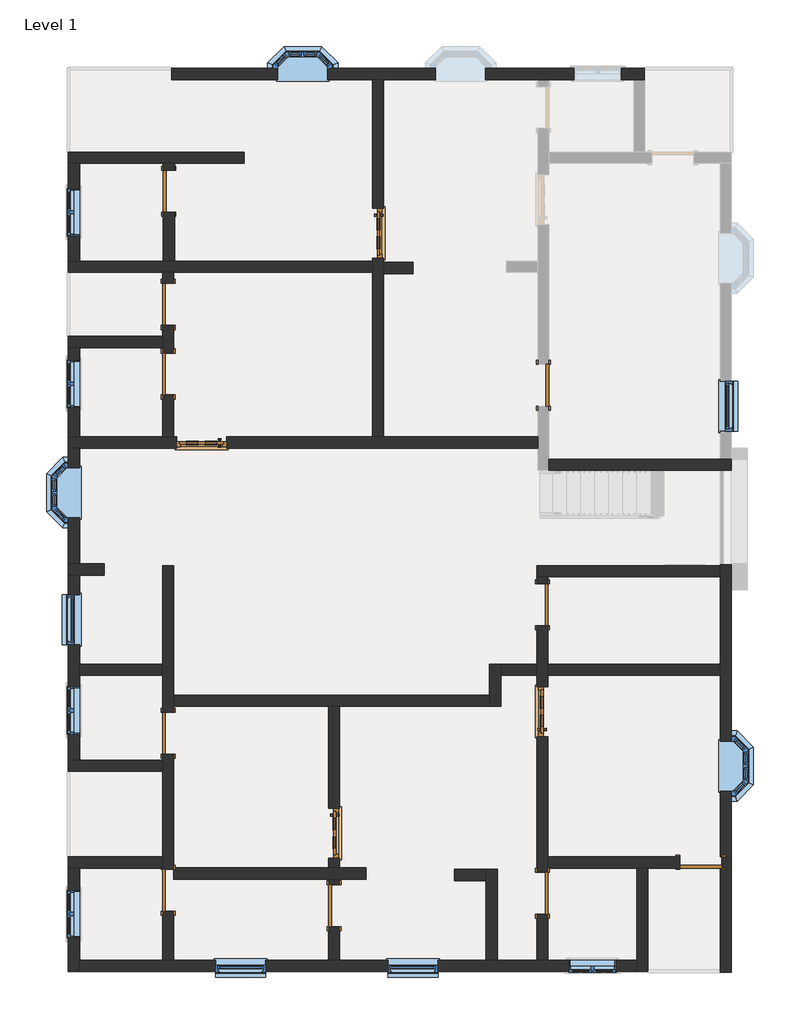
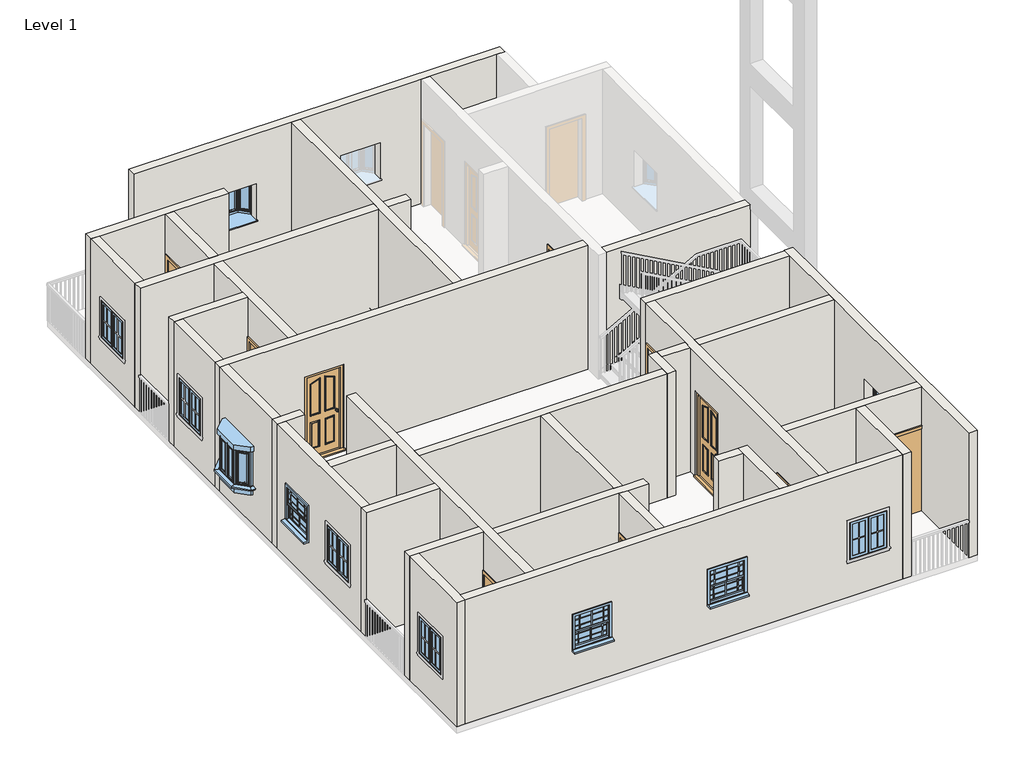
# One storey, part 1 of 4: 34 walls, 14 doors, 12 windows.
"""IFC4 building model written with IfcOpenShell, lengths in millimetres."""

from ifc_helpers import new_model, si_unit, frame, origin, origin_with_axes, place, context, project, spatial, polyline, outline, extrude, faceted_brep, transform, mapped, element, save
from components import doors_extsgl_12_910x2110mm_9a09825e, door_fadea3f2, door_53b1b562, window_910x910mm_67ef725a, window_c29befe5, windows_sash_w_bars_1_910x910mm_b688f793

model = new_model("IFC4")

# Units and contexts
model_context = context("Model", 3, world=origin())
ifc_project = project(units=[si_unit("LENGTHUNIT", "METRE", prefix="MILLI")], contexts=[model_context])

# Site, building, storey
site = spatial("IfcSite", under=ifc_project)
building = spatial("IfcBuilding", under=site)
storey = spatial("IfcBuildingStorey", under=building, Name="Level 1", Elevation=0.0)

# Doors
placement = place(None, origin())
doors_extsgl_12_910x2110mm_shape = doors_extsgl_12_910x2110mm_9a09825e(model_context)
element("IfcDoor", 1, ObjectType="Doors_ExtSgl_12 : 910x2110mm", at=placement, inside=storey, context=model_context, shape_type="MappedRepresentation", body=[
    mapped(doors_extsgl_12_910x2110mm_shape, transform((-1409.2058717, 5320.2339901, 0.0), x_axis=(0.0, -1.0, 0.0), y_axis=(1.0, 0.0, 0.0), z_axis=(0.0, 0.0, 1.0))),
])
element("IfcDoor", 2, ObjectType="Doors_ExtSgl_12 : 910x2110mm", at=placement, inside=storey, context=model_context, shape_type="MappedRepresentation", body=[
    mapped(doors_extsgl_12_910x2110mm_shape, transform((-4622.3058717, 1514.4547293, 0.0), x_axis=(-1.0, 0.0, 0.0), y_axis=(0.0, -1.0, 0.0), z_axis=(0.0, 0.0, 1.0))),
])
element("IfcDoor", 3, ObjectType="Doors_ExtSgl_12 : 910x2110mm", at=placement, inside=storey, context=model_context, shape_type="MappedRepresentation", body=[
    mapped(doors_extsgl_12_910x2110mm_shape, transform((-2209.3058717, -5597.5452707, 0.0), x_axis=(0.0, -1.0, 0.0), y_axis=(1.0, 0.0, 0.0), z_axis=(0.0, 0.0, 1.0))),
])
element("IfcDoor", 4, ObjectType="Doors_ExtSgl_12 : 910x2110mm", at=placement, inside=storey, context=model_context, shape_type="MappedRepresentation", body=[
    mapped(doors_extsgl_12_910x2110mm_shape, transform((1587.9941283, -3384.0437545, 0.0), x_axis=(0.0, 1.0, 0.0), y_axis=(-1.0, 0.0, 0.0), z_axis=(0.0, 0.0, 1.0))),
])
door_shape = door_fadea3f2(model_context)
element("IfcDoor", 5, ObjectType="Single-Flush : 30\" x 80\"", at=placement, inside=storey, context=model_context, shape_type="MappedRepresentation", body=[
    mapped(door_shape, transform((-5219.2058717, 6086.4547293, 0.0), x_axis=(0.0, 1.0, 0.0), y_axis=(-1.0, 0.0, 0.0), z_axis=(0.0, 0.0, 1.0))),
])
element("IfcDoor", 6, ObjectType="Single-Flush : 30\" x 80\"", at=placement, inside=storey, context=model_context, shape_type="MappedRepresentation", body=[
    mapped(door_shape, transform((-5231.9058717, -6637.2703483, 0.0), x_axis=(0.0, 1.0, 0.0), y_axis=(-1.0, 0.0, 0.0), z_axis=(0.0, 0.0, 1.0))),
])
element("IfcDoor", 7, ObjectType="Single-Flush : 30\" x 80\"", at=placement, inside=storey, context=model_context, shape_type="MappedRepresentation", body=[
    mapped(door_shape, transform((-2209.3058717, -6918.3452707, 0.0), x_axis=(0.0, 1.0, 0.0), y_axis=(-1.0, 0.0, 0.0), z_axis=(0.0, 0.0, 1.0))),
])
door_2_shape = door_53b1b562(model_context)
element("IfcDoor", 8, ObjectType="Single-Flush : 30\" x 80\"", at=placement, inside=storey, context=model_context, shape_type="MappedRepresentation", body=[
    mapped(door_2_shape, transform((-5231.9058717, 2759.0547293, 0.0), x_axis=(0.0, -1.0, 0.0), y_axis=(1.0, 0.0, 0.0), z_axis=(0.0, 0.0, 1.0))),
])
element("IfcDoor", 9, ObjectType="Single-Flush : 30\" x 80\"", at=placement, inside=storey, context=model_context, shape_type="MappedRepresentation", body=[
    mapped(door_2_shape, transform((-5231.9058717, -3778.816952, 0.0), x_axis=(0.0, -1.0, 0.0), y_axis=(1.0, 0.0, 0.0), z_axis=(0.0, 0.0, 1.0))),
])
element("IfcDoor", 10, ObjectType="Single-Flush : 30\" x 80\"", at=placement, inside=storey, context=model_context, shape_type="MappedRepresentation", body=[
    mapped(door_2_shape, transform((1587.9941283, -6689.7452707, 0.0), x_axis=(0.0, 1.0, 0.0), y_axis=(-1.0, 0.0, 0.0), z_axis=(0.0, 0.0, 1.0))),
])
element("IfcDoor", 11, ObjectType="Single-Flush : 30\" x 80\"", at=placement, inside=storey, context=model_context, shape_type="MappedRepresentation", body=[
    mapped(door_2_shape, transform((4470.8941283, -6130.9452707, 0.0), x_axis=(1.0, 0.0, 0.0), y_axis=(0.0, 1.0, 0.0), z_axis=(0.0, 0.0, 1.0))),
])
element("IfcDoor", 12, ObjectType="Single-Flush : 30\" x 80\"", at=placement, inside=storey, context=model_context, shape_type="MappedRepresentation", body=[
    mapped(door_2_shape, transform((1587.9941283, -1440.3867138, 0.0), x_axis=(0.0, 1.0, 0.0), y_axis=(-1.0, 0.0, 0.0), z_axis=(0.0, 0.0, 1.0))),
])
element("IfcDoor", 13, ObjectType="Single-Flush : 30\" x 80\"", at=placement, inside=storey, context=model_context, shape_type="MappedRepresentation", body=[
    mapped(door_2_shape, transform((1600.6941283, 2555.8547293, 0.0), x_axis=(0.0, 1.0, 0.0), y_axis=(-1.0, 0.0, 0.0), z_axis=(0.0, 0.0, 1.0))),
])
element("IfcDoor", 14, ObjectType="Single-Flush : 30\" x 80\"", at=placement, inside=storey, context=model_context, shape_type="MappedRepresentation", body=[
    mapped(door_2_shape, transform((-5231.9058717, 4026.9443597, 0.0), x_axis=(0.0, -1.0, 0.0), y_axis=(1.0, 0.0, 0.0), z_axis=(0.0, 0.0, 1.0))),
])

# Walls
element("IfcWall", 15, ObjectType="Generic - 4.5\"", at=placement, inside=storey, context=model_context, shape_type="Brep", body=[
    faceted_brep([(-1510.8058717, 4865.2339901, 2110.0), (-1510.8058717, 4865.2339901, 0.0), (-1510.8058717, 4812.2339901, 0.0), (-1510.8058717, 4609.0339901, 0.0), (-1510.8058717, 1616.0547293, 0.0), (-1510.8058717, 1616.0547293, 3048.0), (-1510.8058717, 4609.0339901, 3048.0), (-1510.8058717, 4812.2339901, 3048.0), (-1510.8058717, 8118.4547293, 3048.0), (-1510.8058717, 8118.4547293, 0.0), (-1510.8058717, 5775.2339901, 0.0), (-1510.8058717, 5775.2339901, 2110.0), (-1307.6058717, 1616.0547293, 0.0), (-1307.6058717, 4587.8547293, 0.0), (-1307.6058717, 4791.0547293, 0.0), (-1307.6058717, 4865.2339901, 0.0), (-1307.6058717, 4865.2339901, 2110.0), (-1307.6058717, 5775.2339901, 2110.0), (-1307.6058717, 5775.2339901, 0.0), (-1307.6058717, 8118.4547293, 0.0), (-1307.6058717, 8118.4547293, 3048.0), (-1307.6058717, 4791.0547293, 3048.0), (-1307.6058717, 4587.8547293, 3048.0), (-1307.6058717, 1616.0547293, 3048.0)], [[[0, 1, 2, 3, 4, 5, 6, 7, 8, 9, 10, 11]], [[12, 13, 14, 15, 16, 17, 18, 19, 20, 21, 22, 23]], [[10, 9, 19, 18]], [[4, 3, 2, 1, 15, 14, 13, 12]], [[8, 7, 6, 5, 23, 22, 21, 20]], [[9, 8, 20, 19]], [[5, 4, 12, 23]], [[18, 17, 11, 10]], [[16, 15, 1, 0]], [[17, 16, 0, 11]]]),
])
element("IfcWall", 16, ObjectType="Generic - 4.5\"", at=placement, inside=storey, context=model_context, shape_type="Brep", body=[
    faceted_brep([(-7048.0058717, 4609.0339901, 0.0), (-5333.5058717, 4609.0339901, 0.0), (-5130.3058717, 4609.0339901, 0.0), (-1510.8058717, 4609.0339901, 0.0), (-1510.8058717, 4609.0339901, 3048.0), (-5130.3058717, 4609.0339901, 3048.0), (-5333.5058717, 4609.0339901, 3048.0), (-7048.0058717, 4609.0339901, 3048.0), (-7048.0058717, 4812.2339901, 0.0), (-7048.0058717, 4812.2339901, 3048.0), (-6844.8058717, 4812.2339901, 3048.0), (-5320.8058717, 4812.2339901, 3048.0), (-5117.6058717, 4812.2339901, 3048.0), (-1510.8058717, 4812.2339901, 3048.0), (-1510.8058717, 4812.2339901, 0.0), (-5117.6058717, 4812.2339901, 0.0), (-5320.8058717, 4812.2339901, 0.0), (-6844.8058717, 4812.2339901, 0.0)], [[[0, 1, 2, 3, 4, 5, 6, 7]], [[8, 9, 10, 11, 12, 13, 14, 15, 16, 17]], [[3, 2, 1, 0, 8, 17, 16, 15, 14]], [[7, 6, 5, 4, 13, 12, 11, 10, 9]], [[4, 3, 14, 13]], [[0, 7, 9, 8]]]),
])
element("IfcWall", 17, ObjectType="Generic - 4.5\"", at=placement, inside=storey, context=model_context, shape_type="Brep", body=[
    faceted_brep([(-5333.5058717, 3645.9443597, 2032.0), (-5333.5058717, 3645.9443597, 0.0), (-5333.5058717, 3444.8547293, 0.0), (-5333.5058717, 3241.6547293, 0.0), (-5333.5058717, 3140.0547293, 0.0), (-5333.5058717, 3140.0547293, 2032.0), (-5333.5058717, 2378.0547293, 2032.0), (-5333.5058717, 2378.0547293, 0.0), (-5333.5058717, 1616.0547293, 0.0), (-5333.5058717, 1616.0547293, 3048.0), (-5333.5058717, 3241.6547293, 3048.0), (-5333.5058717, 3444.8547293, 3048.0), (-5333.5058717, 4609.0339901, 3048.0), (-5333.5058717, 4609.0339901, 0.0), (-5333.5058717, 4407.9443597, 0.0), (-5333.5058717, 4407.9443597, 2032.0), (-5130.3058717, 3140.0547293, 0.0), (-5130.3058717, 3645.9443597, 0.0), (-5130.3058717, 3645.9443597, 2032.0), (-5130.3058717, 4407.9443597, 2032.0), (-5130.3058717, 4407.9443597, 0.0), (-5130.3058717, 4609.0339901, 0.0), (-5130.3058717, 4609.0339901, 3048.0), (-5130.3058717, 1616.0547293, 3048.0), (-5130.3058717, 1616.0547293, 0.0), (-5130.3058717, 2378.0547293, 0.0), (-5130.3058717, 2378.0547293, 2032.0), (-5130.3058717, 3140.0547293, 2032.0)], [[[0, 1, 2, 3, 4, 5, 6, 7, 8, 9, 10, 11, 12, 13, 14, 15]], [[16, 17, 18, 19, 20, 21, 22, 23, 24, 25, 26, 27]], [[8, 7, 25, 24]], [[14, 13, 21, 20]], [[4, 3, 2, 1, 17, 16]], [[12, 11, 10, 9, 23, 22]], [[13, 12, 22, 21]], [[9, 8, 24, 23]], [[26, 25, 7, 6]], [[27, 26, 6, 5]], [[16, 27, 5, 4]], [[18, 17, 1, 0]], [[19, 18, 0, 15]], [[20, 19, 15, 14]]]),
])
element("IfcWall", 18, ObjectType="Generic - 4.5\"", at=placement, inside=storey, context=model_context, shape_type="Brep", body=[
    faceted_brep([(-5130.3058717, -6256.2703483, 2032.0), (-5130.3058717, -6256.2703483, 0.0), (-5130.3058717, -6230.8703483, 0.0), (-5130.3058717, -4159.816952, 0.0), (-5130.3058717, -4159.816952, 2032.0), (-5130.3058717, -3397.816952, 2032.0), (-5130.3058717, -3397.816952, 0.0), (-5130.3058717, -3286.1452707, 0.0), (-5130.3058717, -3082.9452707, 0.0), (-5130.3058717, -733.4452707, 0.0), (-5130.3058717, -733.4452707, 3048.0), (-5130.3058717, -3082.9452707, 3048.0), (-5130.3058717, -3286.1452707, 3048.0), (-5130.3058717, -6230.8703483, 3048.0), (-5130.3058717, -6434.0703483, 3048.0), (-5130.3058717, -7908.9452707, 3048.0), (-5130.3058717, -7908.9452707, 0.0), (-5130.3058717, -7018.2703483, 0.0), (-5130.3058717, -7018.2703483, 2032.0), (-5333.5058717, -4159.816952, 0.0), (-5333.5058717, -4271.4886333, 0.0), (-5333.5058717, -4474.6886333, 0.0), (-5333.5058717, -6029.3452707, 0.0), (-5333.5058717, -6232.5452707, 0.0), (-5333.5058717, -6256.2703483, 0.0), (-5333.5058717, -6256.2703483, 2032.0), (-5333.5058717, -7018.2703483, 2032.0), (-5333.5058717, -7018.2703483, 0.0), (-5333.5058717, -7908.9452707, 0.0), (-5333.5058717, -7908.9452707, 3048.0), (-5333.5058717, -6232.5452707, 3048.0), (-5333.5058717, -6029.3452707, 3048.0), (-5333.5058717, -4474.6886333, 3048.0), (-5333.5058717, -4271.4886333, 3048.0), (-5333.5058717, -2727.3452707, 3048.0), (-5333.5058717, -2524.1452707, 3048.0), (-5333.5058717, -733.4452707, 3048.0), (-5333.5058717, -733.4452707, 0.0), (-5333.5058717, -2524.1452707, 0.0), (-5333.5058717, -2727.3452707, 0.0), (-5333.5058717, -3397.816952, 0.0), (-5333.5058717, -3397.816952, 2032.0), (-5333.5058717, -4159.816952, 2032.0)], [[[0, 1, 2, 3, 4, 5, 6, 7, 8, 9, 10, 11, 12, 13, 14, 15, 16, 17, 18]], [[19, 20, 21, 22, 23, 24, 25, 26, 27, 28, 29, 30, 31, 32, 33, 34, 35, 36, 37, 38, 39, 40, 41, 42]], [[40, 39, 38, 37, 9, 8, 7, 6]], [[17, 16, 28, 27]], [[3, 2, 1, 24, 23, 22, 21, 20, 19]], [[10, 9, 37, 36]], [[15, 14, 13, 12, 11, 10, 36, 35, 34, 33, 32, 31, 30, 29]], [[4, 3, 19, 42]], [[5, 4, 42, 41]], [[6, 5, 41, 40]], [[25, 24, 1, 0]], [[26, 25, 0, 18]], [[27, 26, 18, 17]], [[16, 15, 29, 28]]]),
])
element("IfcWall", 19, ObjectType="Generic - 4.5\"", at=placement, inside=storey, context=model_context, shape_type="Brep", body=[
    faceted_brep([(-7048.0058717, -898.5452707, 0.0), (-6844.8058717, -898.5452707, 0.0), (-6400.7404065, -898.5452707, 0.0), (-6400.7404065, -898.5452707, 3048.0), (-6844.8058717, -898.5452707, 3048.0), (-7048.0058717, -898.5452707, 3048.0), (-7048.0058717, -695.3452707, 0.0), (-7048.0058717, -695.3452707, 3048.0), (-6844.8058717, -695.3452707, 3048.0), (-6400.7404065, -695.3452707, 3048.0), (-6400.7404065, -695.3452707, 0.0), (-6844.8058717, -695.3452707, 0.0)], [[[0, 1, 2, 3, 4, 5]], [[6, 7, 8, 9, 10, 11]], [[2, 1, 0, 6, 11, 10]], [[3, 2, 10, 9]], [[5, 4, 3, 9, 8, 7]], [[0, 5, 7, 6]]]),
])
element("IfcWall", 20, ObjectType="Generic - 4.5\"", at=placement, inside=storey, context=model_context, shape_type="Brep", body=[
    faceted_brep([(-7048.0058717, 6594.4547293, 0.0), (-6844.8058717, 6594.4547293, 0.0), (-5320.8058717, 6594.4547293, 0.0), (-5117.6058717, 6594.4547293, 0.0), (-3847.6058717, 6594.4547293, 0.0), (-3847.6058717, 6594.4547293, 3048.0), (-5117.6058717, 6594.4547293, 3048.0), (-5320.8058717, 6594.4547293, 3048.0), (-6844.8058717, 6594.4547293, 3048.0), (-7048.0058717, 6594.4547293, 3048.0), (-7048.0058717, 6797.6547293, 0.0), (-7048.0058717, 6797.6547293, 3048.0), (-3847.6058717, 6797.6547293, 3048.0), (-3847.6058717, 6797.6547293, 0.0)], [[[0, 1, 2, 3, 4, 5, 6, 7, 8, 9]], [[10, 11, 12, 13]], [[4, 3, 2, 1, 0, 10, 13]], [[5, 4, 13, 12]], [[9, 8, 7, 6, 5, 12, 11]], [[0, 9, 11, 10]]]),
])
element("IfcWall", 21, ObjectType="Generic - 4.5\"", at=placement, inside=storey, context=model_context, shape_type="Brep", body=[
    faceted_brep([(-7048.0058717, 3241.6547293, 0.0), (-6844.8058717, 3241.6547293, 0.0), (-5333.5058717, 3241.6547293, 0.0), (-5333.5058717, 3241.6547293, 3048.0), (-6844.8058717, 3241.6547293, 3048.0), (-7048.0058717, 3241.6547293, 3048.0), (-7048.0058717, 3444.8547293, 0.0), (-7048.0058717, 3444.8547293, 3048.0), (-5333.5058717, 3444.8547293, 3048.0), (-5333.5058717, 3444.8547293, 0.0)], [[[0, 1, 2, 3, 4, 5]], [[6, 7, 8, 9]], [[2, 1, 0, 6, 9]], [[5, 4, 3, 8, 7]], [[3, 2, 9, 8]], [[0, 5, 7, 6]]]),
])
element("IfcWall", 22, ObjectType="Generic - 4.5\"", at=placement, inside=storey, context=model_context, shape_type="Brep", body=[
    faceted_brep([(-7048.0058717, 1412.8547293, 0.0), (-6844.8058717, 1412.8547293, 0.0), (-5077.3058717, 1412.8547293, 0.0), (-5077.3058717, 1412.8547293, 2110.0), (-4167.3058717, 1412.8547293, 2110.0), (-4167.3058717, 1412.8547293, 0.0), (1499.0941283, 1412.8547293, 0.0), (1499.0941283, 1412.8547293, 3048.0), (-6844.8058717, 1412.8547293, 3048.0), (-7048.0058717, 1412.8547293, 3048.0), (-5077.3058717, 1616.0547293, 2110.0), (-5077.3058717, 1616.0547293, 0.0), (-5130.3058717, 1616.0547293, 0.0), (-5333.5058717, 1616.0547293, 0.0), (-6844.8058717, 1616.0547293, 0.0), (-7048.0058717, 1616.0547293, 0.0), (-7048.0058717, 1616.0547293, 3048.0), (-6844.8058717, 1616.0547293, 3048.0), (-5333.5058717, 1616.0547293, 3048.0), (-5130.3058717, 1616.0547293, 3048.0), (-1510.8058717, 1616.0547293, 3048.0), (-1307.6058717, 1616.0547293, 3048.0), (1499.0941283, 1616.0547293, 3048.0), (1499.0941283, 1616.0547293, 0.0), (-1307.6058717, 1616.0547293, 0.0), (-1510.8058717, 1616.0547293, 0.0), (-4167.3058717, 1616.0547293, 0.0), (-4167.3058717, 1616.0547293, 2110.0)], [[[0, 1, 2, 3, 4, 5, 6, 7, 8, 9]], [[10, 11, 12, 13, 14, 15, 16, 17, 18, 19, 20, 21, 22, 23, 24, 25, 26, 27]], [[26, 25, 24, 23, 6, 5]], [[15, 14, 13, 12, 11, 2, 1, 0]], [[9, 8, 7, 22, 21, 20, 19, 18, 17, 16]], [[7, 6, 23, 22]], [[5, 4, 27, 26]], [[3, 2, 11, 10]], [[4, 3, 10, 27]], [[0, 9, 16, 15]]]),
])
element("IfcWall", 23, ObjectType="Generic - 4.5\"", at=placement, inside=storey, context=model_context, shape_type="Brep", body=[
    faceted_brep([(1702.2941283, 1006.4547293, 0.0), (5029.6941283, 1006.4547293, 0.0), (5029.6941283, 1006.4547293, 3048.0), (1702.2941283, 1006.4547293, 3048.0), (1702.2941283, 1209.6547293, 0.0), (1702.2941283, 1209.6547293, 3048.0), (4826.4941283, 1209.6547293, 3048.0), (5029.6941283, 1209.6547293, 3048.0), (5029.6941283, 1209.6547293, 0.0), (4826.4941283, 1209.6547293, 0.0)], [[[0, 1, 2, 3]], [[4, 5, 6, 7, 8, 9]], [[1, 0, 4, 9, 8]], [[3, 2, 7, 6, 5]], [[0, 3, 5, 4]], [[2, 1, 8, 7]]]),
])
element("IfcWall", 24, ObjectType="Generic - 4.5\"", at=placement, inside=storey, context=model_context, shape_type="Brep", body=[
    faceted_brep([(1486.3941283, -932.3867138, 0.0), (1689.5941283, -932.3867138, 0.0), (4826.4941283, -932.3867138, 0.0), (4826.4941283, -932.3867138, 3048.0), (1689.5941283, -932.3867138, 3048.0), (1486.3941283, -932.3867138, 3048.0), (1486.3941283, -729.1867138, 0.0), (1486.3941283, -729.1867138, 3048.0), (4826.4941283, -729.1867138, 3048.0), (4826.4941283, -729.1867138, 0.0)], [[[0, 1, 2, 3, 4, 5]], [[6, 7, 8, 9]], [[2, 1, 0, 6, 9]], [[5, 4, 3, 8, 7]], [[3, 2, 9, 8]], [[0, 5, 7, 6]]]),
])
element("IfcWall", 25, ObjectType="Generic - 4.5\"", at=placement, inside=storey, context=model_context, shape_type="Brep", body=[
    faceted_brep([(1486.3941283, -932.3867138, 0.0), (1486.3941283, -1059.3867138, 0.0), (1486.3941283, -1059.3867138, 2032.0), (1486.3941283, -1821.3867138, 2032.0), (1486.3941283, -1821.3867138, 0.0), (1486.3941283, -2520.4437545, 0.0), (1486.3941283, -2723.6437545, 0.0), (1486.3941283, -2929.0437545, 0.0), (1486.3941283, -2929.0437545, 2110.0), (1486.3941283, -3839.0437545, 2110.0), (1486.3941283, -3839.0437545, 0.0), (1486.3941283, -6308.7452707, 0.0), (1486.3941283, -6308.7452707, 2032.0), (1486.3941283, -7070.7452707, 2032.0), (1486.3941283, -7070.7452707, 0.0), (1486.3941283, -7908.9452707, 0.0), (1486.3941283, -7908.9452707, 3048.0), (1486.3941283, -2723.6437545, 3048.0), (1486.3941283, -2520.4437545, 3048.0), (1486.3941283, -932.3867138, 3048.0), (1689.5941283, -1059.3867138, 2032.0), (1689.5941283, -1059.3867138, 0.0), (1689.5941283, -932.3867138, 0.0), (1689.5941283, -932.3867138, 3048.0), (1689.5941283, -2520.4437545, 3048.0), (1689.5941283, -2723.6437545, 3048.0), (1689.5941283, -6029.3452707, 3048.0), (1689.5941283, -6232.5452707, 3048.0), (1689.5941283, -7908.9452707, 3048.0), (1689.5941283, -7908.9452707, 0.0), (1689.5941283, -7070.7452707, 0.0), (1689.5941283, -7070.7452707, 2032.0), (1689.5941283, -6308.7452707, 2032.0), (1689.5941283, -6308.7452707, 0.0), (1689.5941283, -6232.5452707, 0.0), (1689.5941283, -6029.3452707, 0.0), (1689.5941283, -3839.0437545, 0.0), (1689.5941283, -3839.0437545, 2110.0), (1689.5941283, -2929.0437545, 2110.0), (1689.5941283, -2929.0437545, 0.0), (1689.5941283, -2723.6437545, 0.0), (1689.5941283, -2520.4437545, 0.0), (1689.5941283, -1821.3867138, 0.0), (1689.5941283, -1821.3867138, 2032.0)], [[[0, 1, 2, 3, 4, 5, 6, 7, 8, 9, 10, 11, 12, 13, 14, 15, 16, 17, 18, 19]], [[20, 21, 22, 23, 24, 25, 26, 27, 28, 29, 30, 31, 32, 33, 34, 35, 36, 37, 38, 39, 40, 41, 42, 43]], [[30, 29, 15, 14]], [[36, 35, 34, 33, 11, 10]], [[22, 21, 1, 0]], [[42, 41, 40, 39, 7, 6, 5, 4]], [[19, 18, 17, 16, 28, 27, 26, 25, 24, 23]], [[0, 19, 23, 22]], [[10, 9, 37, 36]], [[8, 7, 39, 38]], [[9, 8, 38, 37]], [[12, 11, 33, 32]], [[13, 12, 32, 31]], [[14, 13, 31, 30]], [[2, 1, 21, 20]], [[3, 2, 20, 43]], [[4, 3, 43, 42]], [[16, 15, 29, 28]]]),
])
element("IfcWall", 26, ObjectType="Generic - 4.5\"", at=placement, inside=storey, context=model_context, shape_type="SweptSolid", body=[
    extrude(outline(polyline([(4826.4941283, -2723.6437545), (1689.5941283, -2723.6437545), (1689.5941283, -2520.4437545), (4826.4941283, -2520.4437545), (4826.4941283, -2723.6437545)])), origin_with_axes(), (0.0, 0.0, 1.0), 3048.0),
])
element("IfcWall", 27, ObjectType="Generic - 4.5\"", at=placement, inside=storey, context=model_context, shape_type="Brep", body=[
    faceted_brep([(4826.4941283, -6232.5452707, 3048.0), (3505.6941283, -6232.5452707, 3048.0), (3302.4941283, -6232.5452707, 3048.0), (1689.5941283, -6232.5452707, 3048.0), (1689.5941283, -6232.5452707, 0.0), (3302.4941283, -6232.5452707, 0.0), (3505.6941283, -6232.5452707, 0.0), (4089.8941283, -6232.5452707, 0.0), (4089.8941283, -6232.5452707, 2032.0), (4826.4941283, -6232.5452707, 2032.0), (1689.5941283, -6029.3452707, 3048.0), (4826.4941283, -6029.3452707, 3048.0), (4826.4941283, -6029.3452707, 2032.0), (4089.8941283, -6029.3452707, 2032.0), (4089.8941283, -6029.3452707, 0.0), (1689.5941283, -6029.3452707, 0.0)], [[[0, 1, 2, 3, 4, 5, 6, 7, 8, 9]], [[10, 11, 12, 13, 14, 15]], [[4, 15, 14, 7, 6, 5]], [[3, 2, 1, 0, 11, 10]], [[11, 0, 9, 12]], [[4, 3, 10, 15]], [[8, 13, 12, 9]], [[13, 8, 7, 14]]]),
])
element("IfcWall", 28, ObjectType="Generic - 4.5\"", at=placement, inside=storey, context=model_context, shape_type="Brep", body=[
    faceted_brep([(3302.4941283, -6232.5452707, 0.0), (3302.4941283, -7908.9452707, 0.0), (3302.4941283, -8112.1452707, 0.0), (3302.4941283, -8112.1452707, 3048.0), (3302.4941283, -7908.9452707, 3048.0), (3302.4941283, -6232.5452707, 3048.0), (3505.6941283, -6232.5452707, 0.0), (3505.6941283, -6232.5452707, 3048.0), (3505.6941283, -8112.1452707, 3048.0), (3505.6941283, -8112.1452707, 0.0)], [[[0, 1, 2, 3, 4, 5]], [[6, 7, 8, 9]], [[2, 1, 0, 6, 9]], [[5, 4, 3, 8, 7]], [[0, 5, 7, 6]], [[3, 2, 9, 8]]]),
])
element("IfcWall", 29, ObjectType="Generic - 4.5\"", at=placement, inside=storey, context=model_context, shape_type="SweptSolid", body=[
    extrude(outline(polyline([(-5333.5058717, -2727.3452707), (-6844.8058717, -2727.3452707), (-6844.8058717, -2524.1452707), (-5333.5058717, -2524.1452707), (-5333.5058717, -2727.3452707)])), origin_with_axes(), (0.0, 0.0, 1.0), 3048.0),
])
element("IfcWall", 30, ObjectType="Generic - 4.5\"", at=placement, inside=storey, context=model_context, shape_type="Brep", body=[
    faceted_brep([(-7048.0058717, -4474.6886333, 0.0), (-5333.5058717, -4474.6886333, 0.0), (-5333.5058717, -4474.6886333, 3048.0), (-7048.0058717, -4474.6886333, 3048.0), (-7048.0058717, -4271.4886333, 0.0), (-7048.0058717, -4271.4886333, 3048.0), (-6844.8058717, -4271.4886333, 3048.0), (-5333.5058717, -4271.4886333, 3048.0), (-5333.5058717, -4271.4886333, 0.0), (-6844.8058717, -4271.4886333, 0.0)], [[[0, 1, 2, 3]], [[4, 5, 6, 7, 8, 9]], [[1, 0, 4, 9, 8]], [[3, 2, 7, 6, 5]], [[2, 1, 8, 7]], [[0, 3, 5, 4]]]),
])
element("IfcWall", 31, ObjectType="Generic - 4.5\"", at=placement, inside=storey, context=model_context, shape_type="Brep", body=[
    faceted_brep([(-7048.0058717, -6232.5452707, 0.0), (-6844.8058717, -6232.5452707, 0.0), (-5333.5058717, -6232.5452707, 0.0), (-5333.5058717, -6232.5452707, 3048.0), (-6844.8058717, -6232.5452707, 3048.0), (-7048.0058717, -6232.5452707, 3048.0), (-7048.0058717, -6029.3452707, 0.0), (-7048.0058717, -6029.3452707, 3048.0), (-5333.5058717, -6029.3452707, 3048.0), (-5333.5058717, -6029.3452707, 0.0)], [[[0, 1, 2, 3, 4, 5]], [[6, 7, 8, 9]], [[2, 1, 0, 6, 9]], [[5, 4, 3, 8, 7]], [[3, 2, 9, 8]], [[0, 5, 7, 6]]]),
])
element("IfcWall", 32, ObjectType="Generic - 4.5\"", at=placement, inside=storey, context=model_context, shape_type="Brep", body=[
    faceted_brep([(-5130.3058717, -6434.0703483, 0.0), (-2310.9058717, -6434.0703483, 0.0), (-2107.7058717, -6434.0703483, 0.0), (-1625.1058717, -6434.0703483, 0.0), (-1625.1058717, -6434.0703483, 3048.0), (-2107.7058717, -6434.0703483, 3048.0), (-2310.9058717, -6434.0703483, 3048.0), (-5130.3058717, -6434.0703483, 3048.0), (-5130.3058717, -6230.8703483, 0.0), (-5130.3058717, -6230.8703483, 3048.0), (-2310.9058717, -6230.8703483, 3048.0), (-2107.7058717, -6230.8703483, 3048.0), (-1625.1058717, -6230.8703483, 3048.0), (-1625.1058717, -6230.8703483, 0.0), (-2107.7058717, -6230.8703483, 0.0), (-2310.9058717, -6230.8703483, 0.0), (-5130.3058717, -6256.2703483, 0.0)], [[[0, 1, 2, 3, 4, 5, 6, 7]], [[8, 9, 10, 11, 12, 13, 14, 15]], [[3, 2, 1, 0, 16, 8, 15, 14, 13]], [[4, 3, 13, 12]], [[7, 6, 5, 4, 12, 11, 10, 9]], [[0, 7, 9, 8, 16]]]),
])
element("IfcWall", 33, ObjectType="Generic - 4.5\"", at=placement, inside=storey, context=model_context, shape_type="Brep", body=[
    faceted_brep([(762.4941283, -7908.9452707, 0.0), (762.4941283, -6257.9452707, 0.0), (762.4941283, -6257.9452707, 3048.0), (762.4941283, -7908.9452707, 3048.0), (559.2941283, -7908.9452707, 0.0), (559.2941283, -7908.9452707, 3048.0), (559.2941283, -6461.1452707, 3048.0), (559.2941283, -6257.9452707, 3048.0), (559.2941283, -6257.9452707, 0.0), (559.2941283, -6461.1452707, 0.0)], [[[0, 1, 2, 3]], [[4, 5, 6, 7, 8, 9]], [[1, 0, 4, 9, 8]], [[3, 2, 7, 6, 5]], [[2, 1, 8, 7]], [[0, 3, 5, 4]]]),
])
element("IfcWall", 34, ObjectType="Generic - 4.5\"", at=placement, inside=storey, context=model_context, shape_type="SweptSolid", body=[
    extrude(outline(polyline([(-12.2058717, -6257.9452707), (559.2941283, -6257.9452707), (559.2941283, -6461.1452707), (-12.2058717, -6461.1452707), (-12.2058717, -6257.9452707)])), origin_with_axes(), (0.0, 0.0, 1.0), 3048.0),
])
element("IfcWall", 35, ObjectType="Generic - 4.5\"", at=placement, inside=storey, context=model_context, shape_type="SweptSolid", body=[
    extrude(outline(polyline([(-3286.1452707, 3048.0), (-3286.1452707, 0.0), (-5142.5452707, 0.0), (-5142.5452707, 2110.0), (-6052.5452707, 2110.0), (-6052.5452707, 0.0), (-6230.8703483, 0.0), (-6230.8703483, 3048.0), (-3286.1452707, 3048.0)])), frame((-2310.9058717, 0.0, 0.0), z_axis=(1.0, 0.0, 0.0), x_axis=(0.0, 1.0, 0.0)), (0.0, 0.0, 1.0), 203.2),
    extrude(outline(polyline([(-6537.3452707, 0.0), (-6537.3452707, 2032.0), (-7299.3452707, 2032.0), (-7299.3452707, 0.0), (-7908.9452707, 0.0), (-7908.9452707, 3048.0), (-6434.0703483, 3048.0), (-6434.0703483, 0.0), (-6537.3452707, 0.0)])), frame((-2310.9058717, 0.0, 0.0), z_axis=(1.0, 0.0, 0.0), x_axis=(0.0, 1.0, 0.0)), (0.0, 0.0, 1.0), 203.2),
])
element("IfcWall", 36, ObjectType="Generic - 4.5\"", at=placement, inside=storey, context=model_context, shape_type="Brep", body=[
    faceted_brep([(-5130.3058717, -3286.1452707, 0.0), (-2310.9058717, -3286.1452707, 0.0), (-2107.7058717, -3286.1452707, 0.0), (622.0199378, -3286.1452707, 0.0), (622.0199378, -3286.1452707, 3048.0), (-2107.7058717, -3286.1452707, 3048.0), (-2310.9058717, -3286.1452707, 3048.0), (-5130.3058717, -3286.1452707, 3048.0), (-5130.3058717, -3082.9452707, 0.0), (-5130.3058717, -3082.9452707, 3048.0), (622.0199378, -3082.9452707, 3048.0), (622.0199378, -3082.9452707, 0.0)], [[[0, 1, 2, 3, 4, 5, 6, 7]], [[8, 9, 10, 11]], [[3, 2, 1, 0, 8, 11]], [[7, 6, 5, 4, 10, 9]], [[0, 7, 9, 8]], [[4, 3, 11, 10]]]),
])
element("IfcWall", 37, ObjectType="Generic - 4.5\"", at=placement, inside=storey, context=model_context, shape_type="Brep", body=[
    faceted_brep([(825.2199378, -3286.1452707, 0.0), (825.2199378, -2723.6437545, 0.0), (825.2199378, -2520.4437545, 0.0), (825.2199378, -2520.4437545, 3048.0), (825.2199378, -2723.6437545, 3048.0), (825.2199378, -3286.1452707, 3048.0), (622.0199378, -3286.1452707, 0.0), (622.0199378, -3286.1452707, 3048.0), (622.0199378, -3082.9452707, 3048.0), (622.0199378, -2520.4437545, 3048.0), (622.0199378, -2520.4437545, 0.0), (622.0199378, -3082.9452707, 0.0)], [[[0, 1, 2, 3, 4, 5]], [[6, 7, 8, 9, 10, 11]], [[2, 1, 0, 6, 11, 10]], [[5, 4, 3, 9, 8, 7]], [[0, 5, 7, 6]], [[3, 2, 10, 9]]]),
])
element("IfcWall", 38, ObjectType="Generic - 4.5\"", at=placement, inside=storey, context=model_context, shape_type="SweptSolid", body=[
    extrude(outline(polyline([(1486.3941283, -2723.6437545), (825.2199378, -2723.6437545), (825.2199378, -2520.4437545), (1486.3941283, -2520.4437545), (1486.3941283, -2723.6437545)])), origin_with_axes(), (0.0, 0.0, 1.0), 3048.0),
])
element("IfcWall", 39, ObjectType="Generic - 4.5\"", at=placement, inside=storey, context=model_context, shape_type="SweptSolid", body=[
    extrude(outline(polyline([(-774.2058717, 4587.8547293), (-1307.6058717, 4587.8547293), (-1307.6058717, 4791.0547293), (-774.2058717, 4791.0547293), (-774.2058717, 4587.8547293)])), origin_with_axes(), (0.0, 0.0, 1.0), 3048.0),
])
element("IfcWall", 40, ObjectType="Generic - 4.5\"", at=placement, inside=storey, context=model_context, shape_type="SweptSolid", body=[
    extrude(outline(polyline([(6594.4547293, 0.0), (6467.4547293, 0.0), (6467.4547293, 2032.0), (5705.4547293, 2032.0), (5705.4547293, 0.0), (4812.2339901, 0.0), (4812.2339901, 3048.0), (6594.4547293, 3048.0), (6594.4547293, 0.0)])), frame((-5320.8058717, 0.0, 0.0), z_axis=(1.0, 0.0, 0.0), x_axis=(0.0, 1.0, 0.0)), (0.0, 0.0, 1.0), 203.2),
])
element("IfcWall", 41, ObjectType="Generic - 9\"", at=placement, inside=storey, context=model_context, shape_type="Brep", body=[
    faceted_brep([(-5168.4058717, 8118.4547293, 0.0), (-1510.8058717, 8118.4547293, 0.0), (-1307.6058717, 8118.4547293, 0.0), (1499.0941283, 8118.4547293, 0.0), (1702.2941283, 8118.4547293, 0.0), (3251.6941283, 8118.4547293, 0.0), (3442.1941283, 8118.4547293, 0.0), (3442.1941283, 8118.4547293, 3048.0), (3251.6941283, 8118.4547293, 3048.0), (1702.2941283, 8118.4547293, 3048.0), (1499.0941283, 8118.4547293, 3048.0), (-1307.6058717, 8118.4547293, 3048.0), (-1510.8058717, 8118.4547293, 3048.0), (-5168.4058717, 8118.4547293, 3048.0), (-359.2558717, 8118.4547293, 1824.4), (550.7441283, 8118.4547293, 1824.4), (550.7441283, 8118.4547293, 914.4), (-359.2558717, 8118.4547293, 914.4), (-3235.8058717, 8118.4547293, 1824.4), (-2325.8058717, 8118.4547293, 1824.4), (-2325.8058717, 8118.4547293, 914.4), (-3235.8058717, 8118.4547293, 914.4), (3023.0941283, 8118.4547293, 1828.8), (3023.0941283, 8118.4547293, 914.4), (2159.4941283, 8118.4547293, 914.4), (2159.4941283, 8118.4547293, 1828.8), (-5168.4058717, 8321.6547293, 0.0), (-5168.4058717, 8321.6547293, 3048.0), (3442.1941283, 8321.6547293, 3048.0), (3442.1941283, 8321.6547293, 0.0), (-359.2558717, 8321.6547293, 1824.4), (-359.2558717, 8321.6547293, 914.4), (550.7441283, 8321.6547293, 914.4), (550.7441283, 8321.6547293, 1824.4), (-3235.8058717, 8321.6547293, 1824.4), (-3235.8058717, 8321.6547293, 914.4), (-2325.8058717, 8321.6547293, 914.4), (-2325.8058717, 8321.6547293, 1824.4), (3023.0941283, 8321.6547293, 1828.8), (2159.4941283, 8321.6547293, 1828.8), (2159.4941283, 8321.6547293, 914.4), (3023.0941283, 8321.6547293, 914.4)], [[[0, 1, 2, 3, 4, 5, 6, 7, 8, 9, 10, 11, 12, 13], [14, 15, 16, 17], [18, 19, 20, 21], [22, 23, 24, 25]], [[26, 27, 28, 29], [30, 31, 32, 33], [34, 35, 36, 37], [38, 39, 40, 41]], [[6, 5, 4, 3, 2, 1, 0, 26, 29]], [[7, 6, 29, 28]], [[13, 12, 11, 10, 9, 8, 7, 28, 27]], [[0, 13, 27, 26]], [[31, 30, 14, 17]], [[32, 31, 17, 16]], [[33, 32, 16, 15]], [[30, 33, 15, 14]], [[35, 34, 18, 21]], [[36, 35, 21, 20]], [[37, 36, 20, 19]], [[34, 37, 19, 18]], [[23, 22, 38, 41]], [[24, 23, 41, 40]], [[25, 24, 40, 39]], [[22, 25, 39, 38]]]),
])
element("IfcWall", 42, ObjectType="Generic - 9\"", at=placement, inside=storey, context=model_context, shape_type="Brep", body=[
    faceted_brep([(4826.4941283, -8124.8452707, 0.0), (4826.4941283, -8124.8452707, 3048.0), (4826.4941283, -6232.5452707, 3048.0), (4826.4941283, -6029.3452707, 3048.0), (4826.4941283, -2723.6437545, 3048.0), (4826.4941283, -2520.4437545, 3048.0), (4826.4941283, -932.3867138, 3048.0), (4826.4941283, -729.1867138, 3048.0), (4826.4941283, -714.2964201, 3048.0), (4826.4941283, -714.2964201, 0.0), (4826.4941283, -729.1867138, 0.0), (4826.4941283, -932.3867138, 0.0), (4826.4941283, -2520.4437545, 0.0), (4826.4941283, -2723.6437545, 0.0), (4826.4941283, -6029.3452707, 0.0), (4826.4941283, -6029.3452707, 2032.0), (4826.4941283, -6232.5452707, 2032.0), (4826.4941283, -6232.5452707, 0.0), (4826.4941283, -3921.4945126, 1824.4), (4826.4941283, -4831.4945126, 1824.4), (4826.4941283, -4831.4945126, 914.4), (4826.4941283, -3921.4945126, 914.4), (5029.6941283, -8124.8452707, 0.0), (5029.6941283, -714.2964201, 0.0), (5029.6941283, -714.2964201, 3048.0), (5029.6941283, -8124.8452707, 3048.0), (5029.6941283, -3921.4945126, 1824.4), (5029.6941283, -3921.4945126, 914.4), (5029.6941283, -4831.4945126, 914.4), (5029.6941283, -4831.4945126, 1824.4), (4851.8941283, -6232.5452707, 0.0), (4851.8941283, -6029.3452707, 0.0), (4851.8941283, -6232.5452707, 2032.0), (4851.8941283, -6029.3452707, 2032.0)], [[[0, 1, 2, 3, 4, 5, 6, 7, 8, 9, 10, 11, 12, 13, 14, 15, 16, 17], [18, 19, 20, 21]], [[22, 23, 24, 25], [26, 27, 28, 29]], [[23, 22, 0, 17, 30, 31, 14, 13, 12, 11, 10, 9]], [[1, 0, 22, 25]], [[8, 7, 6, 5, 4, 3, 2, 1, 25, 24]], [[9, 8, 24, 23]], [[32, 30, 17, 16]], [[31, 33, 15, 14]], [[33, 32, 16, 15]], [[30, 32, 33, 31]], [[27, 26, 18, 21]], [[28, 27, 21, 20]], [[29, 28, 20, 19]], [[26, 29, 19, 18]]]),
])
element("IfcWall", 43, ObjectType="Generic - 9\"", at=placement, inside=storey, context=model_context, shape_type="SweptSolid", body=[
    extrude(outline(polyline([(6594.4547293, 0.0), (4812.2339901, 0.0), (4812.2339901, 3048.0), (6594.4547293, 3048.0), (6594.4547293, 0.0)]), holes=[polyline([(6135.1443597, 1828.8), (5271.5443597, 1828.8), (5271.5443597, 914.4), (6135.1443597, 914.4), (6135.1443597, 1828.8)])]), frame((-7048.0058717, 0.0, 0.0), z_axis=(1.0, 0.0, 0.0), x_axis=(0.0, 1.0, 0.0)), (0.0, 0.0, 1.0), 203.2),
])
element("IfcWall", 44, ObjectType="Generic - 9\"", at=placement, inside=storey, context=model_context, shape_type="SweptSolid", body=[
    extrude(outline(polyline([(3241.6547293, 0.0), (1616.0547293, 0.0), (1616.0547293, 3048.0), (3241.6547293, 3048.0), (3241.6547293, 0.0)]), holes=[polyline([(3013.0547293, 1828.8), (2149.4547293, 1828.8), (2149.4547293, 914.4), (3013.0547293, 914.4), (3013.0547293, 1828.8)])]), frame((-7048.0058717, 0.0, 0.0), z_axis=(1.0, 0.0, 0.0), x_axis=(0.0, 1.0, 0.0)), (0.0, 0.0, 1.0), 203.2),
])
element("IfcWall", 45, ObjectType="Generic - 9\"", at=placement, inside=storey, context=model_context, shape_type="Brep", body=[
    faceted_brep([(-7048.0058717, -898.5452707, 0.0), (-7048.0058717, -4271.4886333, 0.0), (-7048.0058717, -4271.4886333, 3048.0), (-7048.0058717, -898.5452707, 3048.0), (-7048.0058717, -2166.3452707, 914.4), (-7048.0058717, -1256.3452707, 914.4), (-7048.0058717, -1256.3452707, 1824.4), (-7048.0058717, -2166.3452707, 1824.4), (-7048.0058717, -2930.5452707, 1828.8), (-7048.0058717, -3794.1452707, 1828.8), (-7048.0058717, -3794.1452707, 914.4), (-7048.0058717, -2930.5452707, 914.4), (-6844.8058717, -898.5452707, 0.0), (-6844.8058717, -898.5452707, 3048.0), (-6844.8058717, -2524.1452707, 3048.0), (-6844.8058717, -2727.3452707, 3048.0), (-6844.8058717, -4271.4886333, 3048.0), (-6844.8058717, -4271.4886333, 0.0), (-6844.8058717, -2727.3452707, 0.0), (-6844.8058717, -2524.1452707, 0.0), (-6844.8058717, -2166.3452707, 914.4), (-6844.8058717, -2166.3452707, 1824.4), (-6844.8058717, -1256.3452707, 1824.4), (-6844.8058717, -1256.3452707, 914.4), (-6844.8058717, -2930.5452707, 1828.8), (-6844.8058717, -2930.5452707, 914.4), (-6844.8058717, -3794.1452707, 914.4), (-6844.8058717, -3794.1452707, 1828.8)], [[[0, 1, 2, 3], [4, 5, 6, 7], [8, 9, 10, 11]], [[12, 13, 14, 15, 16, 17, 18, 19], [20, 21, 22, 23], [24, 25, 26, 27]], [[1, 0, 12, 19, 18, 17]], [[3, 2, 16, 15, 14, 13]], [[0, 3, 13, 12]], [[2, 1, 17, 16]], [[21, 20, 4, 7]], [[22, 21, 7, 6]], [[23, 22, 6, 5]], [[20, 23, 5, 4]], [[25, 24, 8, 11]], [[26, 25, 11, 10]], [[27, 26, 10, 9]], [[24, 27, 9, 8]]]),
])
element("IfcWall", 46, ObjectType="Generic - 9\"", at=placement, inside=storey, context=model_context, shape_type="Brep", body=[
    faceted_brep([(-7048.0058717, -6232.5452707, 0.0), (-7048.0058717, -8112.1452707, 0.0), (-7048.0058717, -8112.1452707, 3048.0), (-7048.0058717, -6232.5452707, 3048.0), (-7048.0058717, -6638.9452707, 1828.8), (-7048.0058717, -7502.5452707, 1828.8), (-7048.0058717, -7502.5452707, 914.4), (-7048.0058717, -6638.9452707, 914.4), (-6844.8058717, -6232.5452707, 0.0), (-6844.8058717, -6232.5452707, 3048.0), (-6844.8058717, -7908.9452707, 3048.0), (-6844.8058717, -8112.1452707, 3048.0), (-6844.8058717, -8112.1452707, 0.0), (-6844.8058717, -7908.9452707, 0.0), (-6844.8058717, -6638.9452707, 1828.8), (-6844.8058717, -6638.9452707, 914.4), (-6844.8058717, -7502.5452707, 914.4), (-6844.8058717, -7502.5452707, 1828.8)], [[[0, 1, 2, 3], [4, 5, 6, 7]], [[8, 9, 10, 11, 12, 13], [14, 15, 16, 17]], [[1, 0, 8, 13, 12]], [[3, 2, 11, 10, 9]], [[0, 3, 9, 8]], [[2, 1, 12, 11]], [[15, 14, 4, 7]], [[16, 15, 7, 6]], [[17, 16, 6, 5]], [[14, 17, 5, 4]]]),
])
element("IfcWall", 47, ObjectType="Generic - 9\"", at=placement, inside=storey, context=model_context, shape_type="Brep", body=[
    faceted_brep([(-6844.8058717, -8112.1452707, 0.0), (3302.4941283, -8112.1452707, 0.0), (3302.4941283, -8112.1452707, 3048.0), (-6844.8058717, -8112.1452707, 3048.0), (-3456.1058717, -8112.1452707, 914.4), (-4366.1058717, -8112.1452707, 914.4), (-4366.1058717, -8112.1452707, 1824.4), (-3456.1058717, -8112.1452707, 1824.4), (-319.2058717, -8112.1452707, 914.4), (-1229.2058717, -8112.1452707, 914.4), (-1229.2058717, -8112.1452707, 1824.4), (-319.2058717, -8112.1452707, 1824.4), (2064.2441283, -8112.1452707, 1828.8), (2927.8441283, -8112.1452707, 1828.8), (2927.8441283, -8112.1452707, 914.4), (2064.2441283, -8112.1452707, 914.4), (-6844.8058717, -7908.9452707, 0.0), (-6844.8058717, -7908.9452707, 3048.0), (-5333.5058717, -7908.9452707, 3048.0), (-5130.3058717, -7908.9452707, 3048.0), (-2310.9058717, -7908.9452707, 3048.0), (-2107.7058717, -7908.9452707, 3048.0), (559.2941283, -7908.9452707, 3048.0), (762.4941283, -7908.9452707, 3048.0), (1486.3941283, -7908.9452707, 3048.0), (1689.5941283, -7908.9452707, 3048.0), (3302.4941283, -7908.9452707, 3048.0), (3302.4941283, -7908.9452707, 0.0), (1689.5941283, -7908.9452707, 0.0), (1486.3941283, -7908.9452707, 0.0), (762.4941283, -7908.9452707, 0.0), (559.2941283, -7908.9452707, 0.0), (-2107.7058717, -7908.9452707, 0.0), (-2310.9058717, -7908.9452707, 0.0), (-5130.3058717, -7908.9452707, 0.0), (-5333.5058717, -7908.9452707, 0.0), (-3456.1058717, -7908.9452707, 914.4), (-3456.1058717, -7908.9452707, 1824.4), (-4366.1058717, -7908.9452707, 1824.4), (-4366.1058717, -7908.9452707, 914.4), (-319.2058717, -7908.9452707, 914.4), (-319.2058717, -7908.9452707, 1824.4), (-1229.2058717, -7908.9452707, 1824.4), (-1229.2058717, -7908.9452707, 914.4), (2064.2441283, -7908.9452707, 1828.8), (2064.2441283, -7908.9452707, 914.4), (2927.8441283, -7908.9452707, 914.4), (2927.8441283, -7908.9452707, 1828.8)], [[[0, 1, 2, 3], [4, 5, 6, 7], [8, 9, 10, 11], [12, 13, 14, 15]], [[16, 17, 18, 19, 20, 21, 22, 23, 24, 25, 26, 27, 28, 29, 30, 31, 32, 33, 34, 35], [36, 37, 38, 39], [40, 41, 42, 43], [44, 45, 46, 47]], [[1, 0, 16, 35, 34, 33, 32, 31, 30, 29, 28, 27]], [[3, 2, 26, 25, 24, 23, 22, 21, 20, 19, 18, 17]], [[2, 1, 27, 26]], [[0, 3, 17, 16]], [[37, 36, 4, 7]], [[38, 37, 7, 6]], [[39, 38, 6, 5]], [[36, 39, 5, 4]], [[41, 40, 8, 11]], [[42, 41, 11, 10]], [[43, 42, 10, 9]], [[40, 43, 9, 8]], [[45, 44, 12, 15]], [[46, 45, 15, 14]], [[47, 46, 14, 13]], [[44, 47, 13, 12]]]),
])
element("IfcWall", 48, ObjectType="Generic - 9\"", at=placement, inside=storey, context=model_context, shape_type="SweptSolid", body=[
    extrude(outline(polyline([(1412.8547293, 0.0), (-695.3452707, 0.0), (-695.3452707, 3048.0), (1412.8547293, 3048.0), (1412.8547293, 0.0)]), holes=[polyline([(145.0547293, 1824.4), (145.0547293, 914.4), (1055.0547293, 914.4), (1055.0547293, 1824.4), (145.0547293, 1824.4)])]), frame((-7048.0058717, 0.0, 0.0), z_axis=(1.0, 0.0, 0.0), x_axis=(0.0, 1.0, 0.0)), (0.0, 0.0, 1.0), 203.2),
])

# Windows
window_910x910mm_shape = window_910x910mm_67ef725a(model_context)
element("IfcWindow", 49, ObjectType="910x910mm", at=placement, inside=storey, context=model_context, shape_type="MappedRepresentation", body=[
    mapped(window_910x910mm_shape, transform((4919.6375605, -4946.4945126, -285.6), x_axis=(0.0, -1.0, 0.0), y_axis=(1.0, 0.0, 0.0), z_axis=(0.0, 0.0, 1.0))),
])
element("IfcWindow", 50, ObjectType="910x910mm", at=placement, inside=storey, context=model_context, shape_type="MappedRepresentation", body=[
    mapped(window_910x910mm_shape, transform((-2210.8058717, 8211.5981615, -285.6), x_axis=(1.0, 0.0, 0.0), y_axis=(0.0, 1.0, 0.0), z_axis=(0.0, 0.0, 1.0))),
])
element("IfcWindow", 51, ObjectType="910x910mm", at=placement, inside=storey, context=model_context, shape_type="MappedRepresentation", body=[
    mapped(window_910x910mm_shape, transform((-6937.9493039, 1170.0547293, -285.6), x_axis=(0.0, 1.0, 0.0), y_axis=(-1.0, 0.0, 0.0), z_axis=(0.0, 0.0, 1.0))),
])
window_shape = window_c29befe5(model_context)
element("IfcWindow", 52, ObjectType="Window-Casement-Double : 34\" x 36\"", at=placement, inside=storey, context=model_context, shape_type="MappedRepresentation", body=[
    mapped(window_shape, transform((-6946.4058717, 5703.3443597, 0.0), x_axis=(0.0, 1.0, 0.0), y_axis=(-1.0, 0.0, 0.0), z_axis=(0.0, 0.0, 1.0))),
])
element("IfcWindow", 53, ObjectType="Window-Casement-Double : 34\" x 36\"", at=placement, inside=storey, context=model_context, shape_type="MappedRepresentation", body=[
    mapped(window_shape, transform((-6946.4058717, 2581.2547293, 0.0), x_axis=(0.0, 1.0, 0.0), y_axis=(-1.0, 0.0, 0.0), z_axis=(0.0, 0.0, 1.0))),
])
element("IfcWindow", 54, ObjectType="Window-Casement-Double : 34\" x 36\"", at=placement, inside=storey, context=model_context, shape_type="MappedRepresentation", body=[
    mapped(window_shape, transform((2496.0441283, -8010.5452707, 0.0), x_axis=(-1.0, 0.0, 0.0), y_axis=(0.0, -1.0, 0.0), z_axis=(0.0, 0.0, 1.0))),
])
element("IfcWindow", 55, ObjectType="Window-Casement-Double : 34\" x 36\"", at=placement, inside=storey, context=model_context, shape_type="MappedRepresentation", body=[
    mapped(window_shape, transform((-6946.4058717, -7070.7452707, 0.0), x_axis=(0.0, 1.0, 0.0), y_axis=(-1.0, 0.0, 0.0), z_axis=(0.0, 0.0, 1.0))),
])
element("IfcWindow", 56, ObjectType="Window-Casement-Double : 34\" x 36\"", at=placement, inside=storey, context=model_context, shape_type="MappedRepresentation", body=[
    mapped(window_shape, transform((-6946.4058717, -3362.3452707, 0.0), x_axis=(0.0, 1.0, 0.0), y_axis=(-1.0, 0.0, 0.0), z_axis=(0.0, 0.0, 1.0))),
])
windows_sash_w_bars_1_910x910mm_shape = windows_sash_w_bars_1_910x910mm_b688f793(model_context)
element("IfcWindow", 57, ObjectType="Windows_Sash_w-Bars_1 : 910x910mm", at=placement, inside=storey, context=model_context, shape_type="MappedRepresentation", body=[
    mapped(windows_sash_w_bars_1_910x910mm_shape, transform((-3911.1058717, -8010.5452707, 114.4), x_axis=(-1.0, 0.0, 0.0), y_axis=(0.0, -1.0, 0.0), z_axis=(0.0, 0.0, 1.0))),
])
element("IfcWindow", 58, ObjectType="Windows_Sash_w-Bars_1 : 910x910mm", at=placement, inside=storey, context=model_context, shape_type="MappedRepresentation", body=[
    mapped(windows_sash_w_bars_1_910x910mm_shape, transform((-6946.4058717, -1711.3452707, 114.4), x_axis=(0.0, 1.0, 0.0), y_axis=(-1.0, 0.0, 0.0), z_axis=(0.0, 0.0, 1.0))),
])
element("IfcWindow", 59, ObjectType="Windows_Sash_w-Bars_1 : 910x910mm", at=placement, inside=storey, context=model_context, shape_type="MappedRepresentation", body=[
    mapped(windows_sash_w_bars_1_910x910mm_shape, transform((-774.2058717, -8010.5452707, 114.4), x_axis=(-1.0, 0.0, 0.0), y_axis=(0.0, -1.0, 0.0), z_axis=(0.0, 0.0, 1.0))),
])
element("IfcWindow", 60, ObjectType="Windows_Sash_w-Bars_1 : 910x910mm", at=placement, inside=storey, context=model_context, shape_type="MappedRepresentation", body=[
    mapped(windows_sash_w_bars_1_910x910mm_shape, transform((4928.0941283, 2174.8547293, 114.4), x_axis=(0.0, -1.0, 0.0), y_axis=(1.0, 0.0, 0.0), z_axis=(0.0, 0.0, 1.0))),
])

save(model, "model.ifc")

# Revit data of these elements
# Type "Doors_ExtSgl_12 : 910x2110mm"
#   Type Mark = "10"
#   Type Comments = "External Single"
#   Operation = "SingleSwingRight"
#   Construction Type Id = "SGL"
#   Keynote = "L20"
#   Analytic Construction = "Large single-glazed windows"
#   Wrap Layers (Int) from Ext = 0' - 6.98819"
#   Wrap Layers (Ext) from Ext = 0' - 4.03543"
#   Visual Light Transmittance = 0.9
#   Thickness = 0' - 1.73228"
#   Stile Top of Lock rail = 3' - 3.37008"
#   Stile Top Rail = 0' - 5.90551"
#   Stile Shutting = 0' - 4.92126"
#   Stile Muntin Rail = 0' - 4.92126"
#   Stile Lock Rail = 0' - 6.88976"
#   Stile Hanging = 0' - 4.92126"
#   Stile Bottom Rail = 0' - 6.88976"
#   Solar Heat Gain Coefficient = 0.86
#   Rough Width = 2' - 11.82677"
#   Rough Height = 6' - 11.07087"
#   O/A Frame Width = 0' - 2.51969"
#   Heat Transfer Coefficient (U) = 0.979472 BTU/(h·ft²·°F)
#   Handle Z Distance = 3' - 3.37008"
#   Glazing Thickness = 0' - 0.94488"
#   FrameWidth = 0' - 1.65354"
#   FrameOffset - External = 0' - 0.98425"
#   FrameDepth = 0' - 3.50394"
#   Door Panel Width = 2' - 7.77165"
#   Door Panel Thickness = 0' - 1.73228"
#   Door Panel Height = 6' - 6.74016"
#   Cill Thickness = 0' - 2.14567"
#   Cill Projection = 0' - 1.1811"
#   Handle X Distance = 0' - 2.95276"
#   Height = 6' - 11.07087"
#   Structural Tolerance = 0' - 0.25591"
#   Tolerance = 0' - 0.11811"
#   Undercut = 0' - 0.15748"
#   Width = 2' - 11.82677"
#   Cill Extension = 0' - 0.98425"
#   Cavity Closer Width = 0' - 1.9685"
#   Cavity Closer Offset from Ext = 0' - 4.03543"
#   Cavity Closer Depth = 0' - 3.34646"
#   Vis - Ironmongery = yes
#   Vis - Cavity Closers = yes
#   Define Thermal Properties by = 1
#   Function = 1
#   Material Glass = Door - Glazing
#   Material Door = Door - Panel
#   Material Frame = Door - Frame/Mullion
#   Material Ironmongery = Door - Handle
#   Wall Closure = (empty or 0)
# Type "Single-Flush : 30\" x 80\""
#   Type Mark = "5"
#   Construction Type Id = "MDOOR"
#   Assembly Code = "C1020"
#   Analytic Construction = "Metal"
#   Thickness = 0' - 2"
#   Heat Transfer Coefficient (U) = 0.651978 BTU/(h·ft²·°F)
#   Height = 6' - 8"
#   Trim Projection Ext = 0' - 1"
#   Trim Projection Int = 0' - 1"
#   Trim Width = 0' - 3"
#   Width = 2' - 6"
#   Define Thermal Properties by = 1
#   Define Thermal Properties by = 1
#   Door Material = Door - Panel
#   Frame Material = Door - Frame
#   Visual Light Transmittance = 0
#   Solar Heat Gain Coefficient = 0
#   Function = (empty or 0)
#   Wall Closure = (empty or 0)
# Type "Generic - 4.5\""
#   Assembly Code = "B2010"
#   Layers, outside or top first: 0' - 8" no material (function 1)
# Type "Generic - 9\""
#   Assembly Code = "B2010"
#   Layers, outside or top first: 0' - 8" no material (function 1)
# Type "910x910mm"
#   Type Mark = "18"
#   Operation = "UserDefined"
#   Construction Type Id = "GSP4R"
#   Keynote = "L10"
#   Analytic Construction = "1/8 in Pilkington single glazing"
#   Wrap Layers (Ext) from Ext = 0' - 4.03543"
#   Wrap Layers (Int) from Ext = 0' - 6.98819"
#   Window Board Projection = 0' - 0.98425"
#   Window Board Extention = 0' - 0.98425"
#   Visual Light Transmittance = 0.9
#   Solar Heat Gain Coefficient = 0.78
#   Heat Transfer Coefficient (U) = 0.6496 BTU/(h·ft²·°F)
#   Glazing Thickness = 0' - 0.94488"
#   DONT CHANGE - Splay Width = 0' - 7.41997"
#   Rough Width = 2' - 11.82677"
#   Rough Height = 2' - 11.82677"
#   Roof Thickness = 0' - 4.92126"
#   Roof Overhang = 0' - 1.5748"
#   Plinth Thickness = 0' - 6.88976"
#   Height = 2' - 11.82677"
#   Width = 2' - 11.82677"
#   Frame Depth = 0' - 2.55906"
#   Default Head Height = 6' - 11.07087"
#   Cill Depth = 0' - 3.44488"
#   Cavity Closer Width = 0' - 1.9685"
#   Cavity Closer Offset from Ext = 0' - 4.03543"
#   Cavity Closer Depth = 0' - 3.34646"
#   Vis - Cavity Closers = yes
#   Define Thermal Properties by = 1
#   Material Trim = Window Frame
#   Material Glass = Glass
#   Material Frame = Window Frame
#   Manufacturer = ""
#   Wall Closure = (empty or 0)
# Type "Window-Casement-Double : 34\" x 36\""
#   Type Mark = "14"
#   Fire Rating = "0.5h"
#   Assembly Code = "B2020100"
#   Analytic Construction = "Double glazing - domestic"
#   Frame Extension [instance default] = 0' - 0 1/4"
#   Window Inset [instance default] = 0' - 0"
#   Wall Thickness [instance default] = 0' - 6"
#   Interior Wall Closure [instance default] = 0' - 2 1/4"
#   Half Width = 1' - 5"
#   Visual Light Transmittance = 0.81
#   Thermal Resistance (R) = 1.8146 (h·ft²·°F)/BTU
#   Solar Heat Gain Coefficient = 0.76
#   Rough Width = 2' - 10 1/2"
#   Rough Height = 3' - 0 1/2"
#   Height = 3' - 0"
#   Heat Transfer Coefficient (U) = 0.5511 BTU/(h·ft²·°F)
#   Exterior Wall Closure [instance default] = 0' - 1 1/4"
#   Extension Jamb [instance default] = 0' - 2 1/4"
#   Default Sill Height = 3' - 0"
#   Width = 2' - 10"
#   Define Thermal Properties by = 0
#   Muntin Visibility = yes
#   Interior Trim Visibility [instance default] = yes
#   Exterior Trim Visibility [instance default] = yes
#   Extension Jamb Visibility [instance default] = yes
#   Interior Trim Material = Wood - Stained
#   Muntin Pattern = Muntin Pattern_2x2 : Muntin Pattern_2x2
#   Interior Trim = Trim-Window-Interior-Flat : Picture Frame
#   Interior Frame Material = Wood - Stained
#   Glass Panel Material = Glass
#   Exterior Trim Material = Clad - White
#   Exterior Trim = Trim-Window-Exterior-Flat : with Sill
#   Exterior Frame Material = Clad - White
#   Wall Closure = (empty or 0)
# Type "Windows_Sash_w-Bars_1 : 910x910mm"
#   Type Mark = "24"
#   Construction Type Id = "GSP4R"
#   Analytic Construction = "1/8 in Pilkington single glazing"
#   Wrap Layers (Int) from Ext = 0' - 6.98819"
#   Wrap Layers (Ext) from Ext = 0' - 4.03543"
#   Window Board Projection = 0' - 0.98425"
#   Window Board Extension = 0' - 0.98425"
#   Visual Light Transmittance = 0.9
#   Solar Heat Gain Coefficient = 0.78
#   Rough Width = 2' - 11.82677"
#   Rough Height = 2' - 11.82677"
#   Height = 2' - 11.82677"
#   Heat Transfer Coefficient (U) = 0.6496 BTU/(h·ft²·°F)
#   Glazing Thickness = 0' - 0.94488"
#   Glazing Bar Offset = 0' - 3.93701"
#   Frame Depth = 0' - 3.54331"
#   FrameOffset - External = 0' - 1.9685"
#   Default Sill Height = 2' - 7.49606"
#   Width = 2' - 11.82677"
#   Glazing Bar Thickness = 0' - 0.7874"
#   Cavity Closer Width = 0' - 1.9685"
#   Cavity Closer Offset from Ext = 0' - 4.03543"
#   Cavity Closer Depth = 0' - 3.34646"
#   Vis - Vert Bar Top = yes
#   Vis - Vert Bar Bttm = yes
#   Vis - Glazing Bars Top = yes
#   Vis - Glazing Bars Bttm = yes
#   Vis - Cavity Closers = yes
#   Define Thermal Properties by = 1
#   Material Trim = Window Frame
#   Material Frame = Window Frame
#   Material Glazing Bars = Window Frame
#   Material Glass = Glass
#   Wall Closure = (empty or 0)
# Elements 1, 2, 3, 4 (IfcDoor, "Doors_ExtSgl_12 : 910x2110mm")
#   Phase Created = New Construction
#   Materials on its faces: "Door - Panel", "Door - Handle", "Door - Frame/Mullion", "Door - Glazing"
# Elements 5, 6, 7, 8, 9, 10, 11, 12, 13, 14 (IfcDoor, "Single-Flush : 30\" x 80\"")
#   Phase Created = New Construction
#   Materials on its faces: "Door - Frame", "Door - Panel"
# Elements 15, 17, 18 (IfcWall, "Generic - 4.5\"")
#   Top Offset = 0' - 0"
#   Base Offset = 0' - 0"
#   wall height = 10' - 0"
#   Phase Created = New Construction
#   Base Constraint = Level 1
#   Top Constraint = Level 2
#   Materials on its faces: "Default Wall", "Brick, Soldier Course"
# Elements 16, 20, 27, 31 (IfcWall, "Generic - 4.5\"")
#   Top Offset = 0' - 0"
#   Base Offset = 0' - 0"
#   wall height = 10' - 0"
#   Phase Created = New Construction
#   Base Constraint = Level 1
#   Top Constraint = Level 2
#   Materials on its faces: "Default Wall", "Parking Stripe"
# Elements 19, 21, 22, 30 (IfcWall, "Generic - 4.5\"")
#   Top Offset = 0' - 0"
#   Base Offset = 0' - 0"
#   wall height = 10' - 0"
#   Phase Created = New Construction
#   Base Constraint = Level 1
#   Top Constraint = Level 2
#   Materials on its faces: "Default Wall", "Earth"
